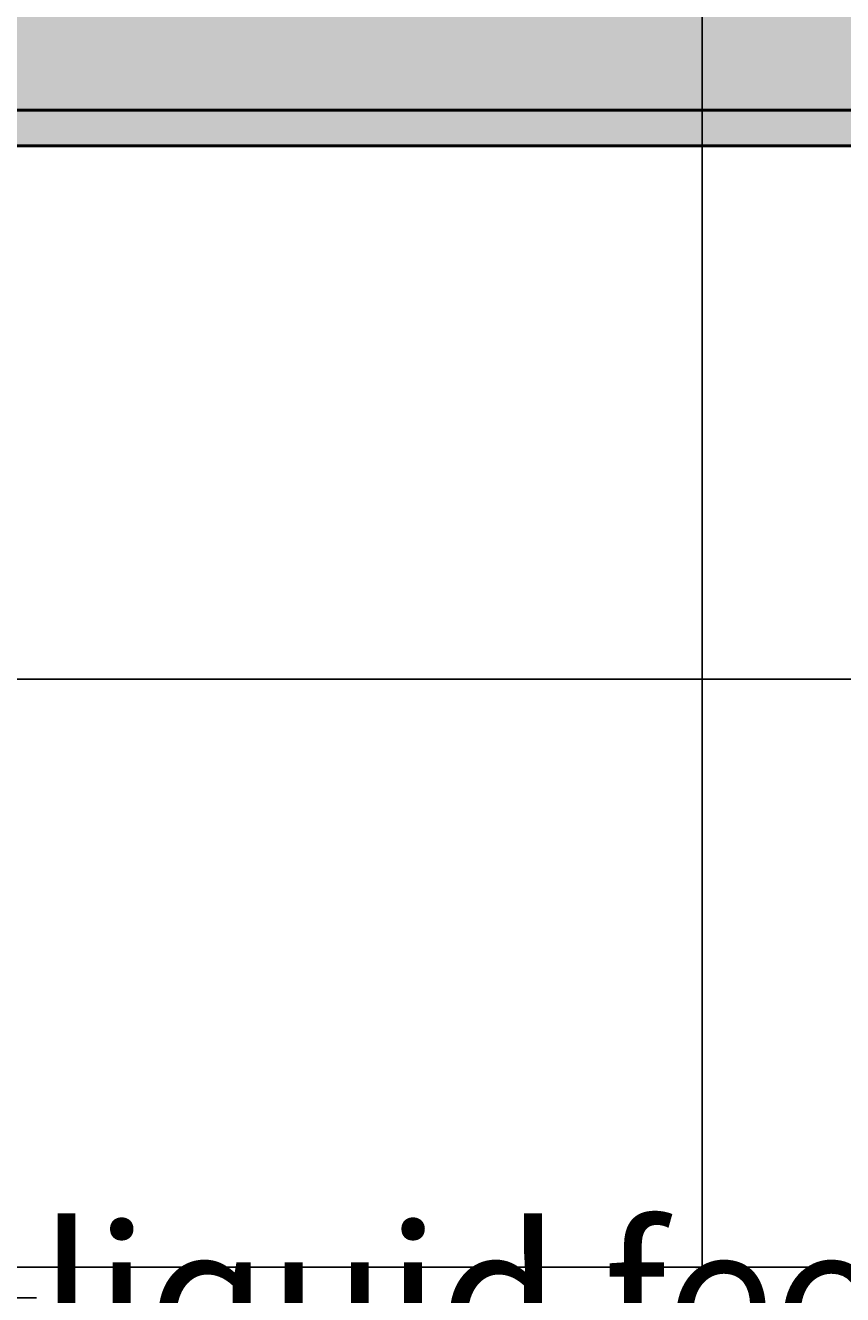
# Model space of a CAD drawing. Units: inches. Extents: x -12 to 334, y -10 to 186.
# Tile 33 of 77: x 152 to 175, y 14 to 49. Entities that reach past the tile are written whole.
import ezdxf
from ezdxf import colors
from ezdxf.entities.mleader import LeaderData, LeaderLine
from ezdxf.math import Vec2, Vec3

# ---------------------------------------------------------------- set-up
doc = ezdxf.new("R2010")
doc.units = ezdxf.units.IN
doc.header["$MEASUREMENT"] = 0
for name, color, linetype, lineweight in [('M-ANNO-TEXT', 3, 'Continuous', 25), ('M-DIMS', 2, 'Continuous', 18), ('M-EQPM', 7, 'Continuous', 50), ('M-EQPM-PATT', 8, 'Continuous', 18)]:
    doc.layers.add(name, color=color, linetype=linetype, lineweight=lineweight)
doc.styles.get("Standard").update_dxf_attribs({"font": 'arial.ttf'})
doc.dimstyles.get("Standard").update_dxf_attribs({"dimtxt": 0.18, "dimasz": 0.18, "dimexe": 0.18, "dimexo": 0.0625, "dimgap": 0.09, "dimtad": 0, "dimtih": 1, "dimtoh": 1, "dimdec": 4, "dimzin": 0, "dimdsep": 46, "dimtxsty": 'Standard', "dimcen": 0.09, "dimadec": 0, "dimazin": 0, "dimtfac": 1, "dimtdec": 4, "dimtofl": 0, "dimtmove": 0, "dimatfit": 3, "dimfxl": 1, "dimtolj": 1, "dimtzin": 0, "dimarcsym": 0})

# ---------------------------------------------------------------- blocks, each defined once
blk = doc.blocks.new('*D1')
at = {"layer": 'Defpoints', "color": 0, "transparency": 16777216}
for p in [(281.426, 91.899), (3.376, 80.692), (281.426, 14.304)]:
    blk.add_point(p, dxfattribs=at)
at = {"layer": 'M-DIMS', "color": 0, "lineweight": -2, "transparency": 16777216}
for p, q in [((281.426, 91.836), (281.426, 14.124)), ((3.376, 80.629), (3.376, 14.124)), ((3.556, 14.304), (141.935, 14.304)), ((281.246, 14.304), (142.867, 14.304))]:
    blk.add_line(p, q, dxfattribs=at)
at = {"layer": 'M-DIMS', "color": 0, "transparency": 16777216}
for points in [[(3.556, 14.334), (3.556, 14.274), (3.376, 14.304)], [(281.246, 14.334), (281.246, 14.274), (281.426, 14.304)]]:
    blk.add_solid(points, dxfattribs=at)
at = {"layer": 'M-DIMS', "color": 0, "transparency": 16777216, "insert": (142.401, 14.304), "char_height": 0.18, "attachment_point": 5}
blk.add_mtext('\\A1;278.05', dxfattribs=at)
blk = doc.blocks.new('*D29')
at = {"layer": 'Defpoints', "color": 0, "transparency": 16777216}
for p in [(-11.174, 45.854), (221.576, 45.854), (216.576, 30.854)]:
    blk.add_point(p, dxfattribs=at)
at = {"layer": 'M-DIMS', "color": 0, "lineweight": -2, "transparency": 16777216}
for p, q in [((221.514, 45.854), (-11.354, 45.854)), ((-11.174, 45.674), (-11.174, 38.536)), ((-11.174, 31.034), (-11.174, 38.172)), ((216.514, 30.854), (-11.354, 30.854))]:
    blk.add_line(p, q, dxfattribs=at)
at = {"layer": 'M-DIMS', "color": 0, "transparency": 16777216}
for points in [[(-11.204, 45.674), (-11.144, 45.674), (-11.174, 45.854)], [(-11.204, 31.034), (-11.144, 31.034), (-11.174, 30.854)]]:
    blk.add_solid(points, dxfattribs=at)
at = {"layer": 'M-DIMS', "color": 0, "transparency": 16777216, "insert": (-11.174, 38.354), "char_height": 0.18, "attachment_point": 5}
blk.add_mtext('\\A1;15', dxfattribs=at)
blk = doc.blocks.new('*D31')
at = {"layer": 'Defpoints', "color": 0, "transparency": 16777216}
for p in [(129.093, 61.105), (170.908, 61.105), (170.908, 14.304)]:
    blk.add_point(p, dxfattribs=at)
at = {"layer": 'M-DIMS', "color": 0, "lineweight": -2, "transparency": 16777216}
for p, q in [((129.093, 61.042), (129.093, 14.124)), ((170.908, 61.042), (170.908, 14.124)), ((129.273, 14.304), (149.532, 14.304)), ((170.728, 14.304), (150.468, 14.304))]:
    blk.add_line(p, q, dxfattribs=at)
at = {"layer": 'M-DIMS', "color": 0, "transparency": 16777216}
for points in [[(129.273, 14.334), (129.273, 14.274), (129.093, 14.304)], [(170.728, 14.334), (170.728, 14.274), (170.908, 14.304)]]:
    blk.add_solid(points, dxfattribs=at)
at = {"layer": 'M-DIMS', "color": 0, "transparency": 16777216, "insert": (150, 14.304), "char_height": 0.18, "attachment_point": 5}
blk.add_mtext('\\A1;41.815', dxfattribs=at)
blk = doc.blocks.new('*D32')
at = {"layer": 'Defpoints', "color": 0, "transparency": 16777216}
for p in [(170.908, 61.105), (216.428, 61.105), (216.428, 14.304)]:
    blk.add_point(p, dxfattribs=at)
at = {"layer": 'M-DIMS', "color": 0, "lineweight": -2, "transparency": 16777216}
for p, q in [((170.908, 61.042), (170.908, 14.124)), ((216.428, 61.042), (216.428, 14.124)), ((171.088, 14.304), (193.271, 14.304)), ((216.248, 14.304), (194.064, 14.304))]:
    blk.add_line(p, q, dxfattribs=at)
at = {"layer": 'M-DIMS', "color": 0, "transparency": 16777216}
for points in [[(171.088, 14.334), (171.088, 14.274), (170.908, 14.304)], [(216.248, 14.334), (216.248, 14.274), (216.428, 14.304)]]:
    blk.add_solid(points, dxfattribs=at)
at = {"layer": 'M-DIMS', "color": 0, "transparency": 16777216, "insert": (193.668, 14.304), "char_height": 0.18, "attachment_point": 5}
blk.add_mtext('\\A1;45.52', dxfattribs=at)
blk = doc.blocks.new('*D39')
at = {"layer": 'Defpoints', "color": 0, "transparency": 16777216}
for p in [(279.726, 80.692), (-11.174, 45.854), (269.381, 45.854)]:
    blk.add_point(p, dxfattribs=at)
at = {"layer": 'M-DIMS', "color": 0, "lineweight": -2, "transparency": 16777216}
for p, q in [((279.664, 80.692), (-11.354, 80.692)), ((-11.174, 80.512), (-11.174, 63.455)), ((-11.174, 46.034), (-11.174, 63.091)), ((269.318, 45.854), (-11.354, 45.854))]:
    blk.add_line(p, q, dxfattribs=at)
at = {"layer": 'M-DIMS', "color": 0, "transparency": 16777216}
for points in [[(-11.204, 80.512), (-11.144, 80.512), (-11.174, 80.692)], [(-11.204, 46.034), (-11.144, 46.034), (-11.174, 45.854)]]:
    blk.add_solid(points, dxfattribs=at)
at = {"layer": 'M-DIMS', "color": 0, "transparency": 16777216, "insert": (-11.174, 63.273), "char_height": 0.18, "attachment_point": 5}
blk.add_mtext('\\A1;34.84', dxfattribs=at)

msp = doc.modelspace()

# ---------------------------------------------------------------- hatches: boundary and pattern name
at = {"layer": 'M-EQPM-PATT'}
h = msp.add_hatch(color=256, dxfattribs=at)
h.set_gradient(color1=(99, 100, 102), color2=(99, 100, 102), tint=1)
h.paths.add_polyline_path([(4.3766, 80.754, -0.4132606), (23.5807, 99.8958), (37.1002, 99.8958), (37.1002, 127.7078), (32.1002, 127.7078), (32.1002, 125.2078), (36.1002, 125.2078), (36.1002, 100.8958), (23.5807, 100.8958, 1), (23.5807, 60.4872), (36.1002, 60.4872), (36.1002, 36.1752), (32.1002, 36.1752), (32.1002, 33.6752), (37.1002, 33.6752), (37.1002, 61.4872), (23.5807, 61.4872, -0.384914), (4.4744, 78.754), (72.9244, 78.754), (72.9244, 69.6117), (75.9244, 69.6117), (75.9244, 89.8963), (72.9244, 89.8963), (72.9244, 80.754)])
h.paths.add_polyline_path([(54.1002, 125.2078), (58.1002, 125.2078), (58.1002, 127.7078), (53.1002, 127.7078), (53.1002, 99.8958), (64.5, 99.8958), (64.5, 109.0583), (63.5, 109.0583), (63.5, 100.8958), (54.1002, 100.8958)], flags=17)
h.paths.add_polyline_path([(53.1002, 33.6752), (58.1002, 33.6752), (58.1002, 36.1752), (54.1002, 36.1752), (54.1002, 60.4872), (64.2068, 60.4872), (64.2068, 49.4497), (87.8879, 49.4497), (87.8879, 55.3205), (104.8919, 55.3205), (104.8919, 30.8541), (99.8919, 30.8541), (99.8919, 28.8541), (105.8919, 28.8541), (105.8919, 56.3205), (87.8879, 56.3205), (87.8879, 63.6117), (86.8879, 63.6117), (86.8879, 50.4497), (65.0061, 50.4497), (65.0061, 63.6117), (64.5, 63.6117), (64.5, 61.4872), (53.1002, 61.4872)])
h.paths.add_polyline_path([(121.8919, 28.8541), (121.8919, 30.8541), (116.8919, 30.8541), (116.8919, 45.8541), (209.6965, 45.8541), (209.9204, 46.8541), (115.8919, 46.8541), (115.8919, 28.8541)])
h.paths.add_polyline_path([(221.5761, 32.8541), (216.5761, 32.8541), (216.5761, 30.8541), (222.5761, 30.8541), (222.5761, 46.8541), (209.9204, 46.8541), (209.6965, 45.8541), (221.5761, 45.8541)])
h.paths.add_polyline_path([(233.5761, 45.8541), (249.8485, 45.8541), (249.3759, 46.8541), (232.5761, 46.8541), (232.5761, 30.8541), (238.5761, 30.8541), (238.5761, 32.8541), (233.5761, 32.8541)])
h = msp.add_hatch(color=256, dxfattribs=at)
h.set_gradient(color1=(94, 103, 175), color2=(94, 103, 175), tint=1)
h.paths.add_polyline_path([(129.093, 89.8963), (86.8879, 89.8963), (86.8879, 69.6117), (129.093, 69.6117)], flags=17)
h.paths.add_polyline_path([(170.9079, 89.8963), (130.8573, 89.8963), (130.8573, 69.6117), (170.9079, 69.6117)], flags=17)
h.paths.add_polyline_path([(216.4278, 89.8963), (172.6722, 89.8963), (172.6722, 69.6117), (216.4278, 69.6117)], flags=17)
h.paths.add_polyline_path([(245.9354, 82.6969), (247.9354, 82.6969), (247.9354, 46.8541), (268.3808, 46.8541, 0.0998398), (279.7263, 80.6915), (251.9801, 80.6915, 0.4142136), (231.7758, 100.8958), (84.7229, 100.8958), (84.7229, 109.0583), (83.7229, 109.0583), (83.7229, 95.8963), (129.093, 95.8963), (129.093, 98.1081), (130.8573, 98.1081), (130.8573, 95.8963), (170.9079, 95.8963), (170.9079, 98.1081), (172.6722, 98.1081), (172.6722, 95.8963), (216.4278, 95.8963), (216.4278, 98.1081), (218.1922, 98.1081), (218.1922, 95.8963), (226.6083, 95.8963, -1), (226.6083, 63.6117), (218.1922, 63.6117), (218.1922, 61.1045), (216.4278, 61.1045), (216.4278, 63.6117), (172.6722, 63.6117), (172.6722, 61.1045), (170.9079, 61.1045), (170.9079, 63.6117), (130.8573, 63.6117), (130.8573, 61.1045), (129.093, 61.1045), (129.093, 63.6117), (87.8879, 63.6117), (87.8879, 56.3205), (105.8919, 56.3205), (105.8919, 28.8541), (115.8919, 28.8541), (115.8919, 46.8541), (222.5761, 46.8541), (222.5761, 30.8541), (232.5761, 30.8541), (232.5761, 46.8541), (245.9354, 46.8541)])
h.paths.add_polyline_path([(86.8879, 89.8963), (75.9244, 89.8963), (75.9244, 69.6117), (86.8879, 69.6117)])
h.paths.add_polyline_path([(83.7229, 109.0583), (75.9244, 109.0583), (75.9244, 95.8963), (83.7229, 95.8963)])
h.paths.add_polyline_path([(226.6083, 89.8963), (218.1922, 89.8963), (218.1922, 69.6117), (226.6083, 69.6117, 1)], flags=17)
h = msp.add_hatch(color=256, dxfattribs=at)
h.set_gradient(color1=(0, 0, 255), color2=(0, 0, 255), tint=1)
h.paths.add_polyline_path([(84.7229, 100.8958), (84.7229, 109.0583), (83.7229, 109.0583), (83.7229, 95.8963), (129.093, 95.8963), (129.093, 98.1081), (130.8573, 98.1081), (130.8573, 95.8963), (170.9079, 95.8963), (170.9079, 98.1081), (172.6722, 98.1081), (172.6722, 95.8963), (216.4278, 95.8963), (216.4278, 98.1081), (218.1922, 98.1081), (218.1922, 95.8963), (226.6083, 95.8963, -1), (226.6083, 63.6117), (218.1922, 63.6117), (218.1922, 61.1045), (216.4278, 61.1045), (216.4278, 63.6117), (172.6722, 63.6117), (172.6722, 61.1045), (170.9079, 61.1045), (170.9079, 63.6117), (130.8573, 63.6117), (130.8573, 61.1045), (129.093, 61.1045), (129.093, 63.6117), (87.8879, 63.6117), (87.8879, 56.3205), (105.8919, 56.3205), (105.8919, 28.8541), (115.8919, 28.8541), (115.8919, 46.8541), (222.5761, 46.8541), (222.5761, 30.8541), (232.5761, 30.8541), (232.5761, 46.8541), (245.9354, 46.8541), (245.9354, 82.6969), (247.9354, 82.6969), (247.9354, 46.8541), (268.3808, 46.8541, 0.0998398), (279.7263, 80.6915), (251.9801, 80.6915, 0.4142136), (231.7758, 100.8958)])

# ---------------------------------------------------------------- linework, layer by layer
at = {"layer": 'M-EQPM'}
for p, q in [((222.5761, 46.8541), (115.8919, 46.8541)), ((221.5761, 45.8541), (116.8919, 45.8541))]:
    msp.add_line(p, q, dxfattribs=at)

# ---------------------------------------------------------------- dimensions: what is measured, and where the dimension line sits
at = {"layer": 'M-DIMS'}
for base, p1, p2, override, picture, middle in [((281.4256, 14.3041), (3.3765, 80.6915), (281.4256, 91.8988), {"dimdec": 2, "dimlfac": 1, "dimrnd": 0, "dimzin": 0, "dimdsep": 46, "dimlunit": 2}, '*D1', (142.401, 14.3041)), ((170.9079, 14.3041), (129.093, 61.1045), (170.9079, 61.1045), {"dimdec": 3, "dimlfac": 1, "dimrnd": 0, "dimzin": 0, "dimdsep": 46, "dimlunit": 2}, '*D31', (150.0004, 14.3041)), ((216.4278, 14.3041), (170.9079, 61.1045), (216.4278, 61.1045), {"dimdec": 2, "dimlfac": 1, "dimrnd": 0, "dimzin": 0, "dimdsep": 46, "dimlunit": 2}, '*D32', (193.6678, 14.3041))]:
    dim = msp.add_linear_dim(base=base, p1=p1, p2=p2, dimstyle='Standard', override=override, dxfattribs=at)
    dim.commit()
    dim.dimension.update_dxf_attribs({"geometry": picture, "text_midpoint": middle})
for p1, p2, override, picture, middle in [((279.7263, 80.6915), (269.3808, 45.8541), {"dimdec": 2, "dimlfac": 1, "dimrnd": 0, "dimzin": 0, "dimdsep": 46, "dimlunit": 2}, '*D39', (-11.1735, 63.2728)), ((216.5761, 30.8541), (221.5761, 45.8541), {"dimdec": 0, "dimlfac": 1, "dimrnd": 0, "dimzin": 0, "dimdsep": 46, "dimlunit": 2}, '*D29', (-11.1735, 38.3541))]:
    dim = msp.add_linear_dim(base=(-11.1736, 45.8541), p1=p1, p2=p2, angle=90, dimstyle='Standard', override=override, dxfattribs=at)
    dim.commit()
    dim.dimension.update_dxf_attribs({"geometry": picture, "text_midpoint": middle})

# ---------------------------------------------------------------- leaders
at = {"layer": 'M-ANNO-TEXT'}
ml = msp.add_multileader_mtext('Standard', dxfattribs=at)
ml.set_content('liquid feed from\\Pcolumn', color=256)
ml.set_leader_properties()
ml.build(insert=Vec2(0, 0))
ml.multileader.update_dxf_attribs({"dogleg_length": 0.36, "arrow_head_size": 0.7})
ctx = ml.context
ctx.base_point, ctx.arrow_head_size, ctx.landing_gap_size, ctx.plane_origin = Vec3(152.1867, 13.4469), 0.7, 0.09, Vec3(117.7335, 28.8541)
notes = []
notes.append((ctx, [(0, (1, 1, 0), (139.1325, 13.4469), (1, 0), 13.0542, [(0, [(117.7335, 28.8541)], 0, [])])]))
ctx.mtext.insert, ctx.mtext.flow_direction = Vec3(152.2767, 15.4796), 5
for ctx, leaders in notes:
    for number, flags, end, landing, length, lines in leaders:
        leader = LeaderData()
        leader.index, (leader.has_last_leader_line, leader.has_dogleg_vector, leader.attachment_direction) = number, flags
        leader.last_leader_point, leader.dogleg_vector, leader.dogleg_length = Vec3(end), Vec3(landing), length
        for number, points, colour, breaks in lines:
            line = LeaderLine()
            line.index, line.vertices, line.color, line.breaks = number, Vec3.list(points), colors.encode_raw_color(colour), breaks
            leader.lines.append(line)
        ctx.leaders.append(leader)

doc.saveas('drawing.dxf')
